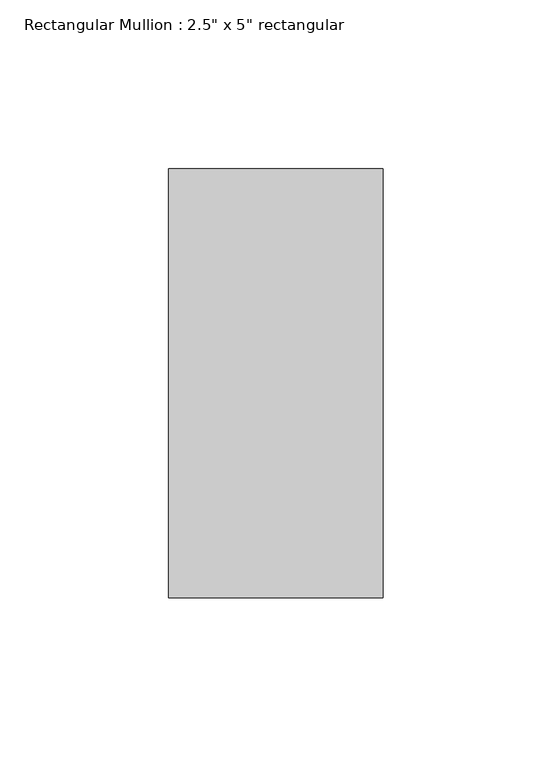
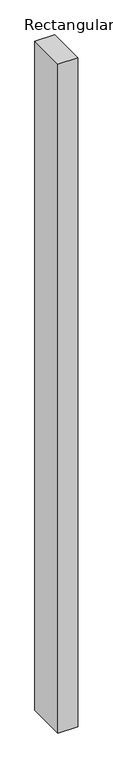
"""IFC4 building model written with IfcOpenShell, lengths in millimetres: member geometry."""

from ifc_helpers import new_model, si_unit, frame, origin, place, context, project, spatial, polyline, outline, extrude, source, transform, mapped, element, save


def member_d9e57c59(model_context):
    return source(origin(), model_context, "Body", "SweptSolid", [
        extrude(outline(polyline([(0.0, 63.5), (0.0, -63.5), (-63.5, -63.5), (-63.5, 63.5), (0.0, 63.5)])), frame((0.0, 0.0, -2256.3666667), z_axis=(0.0, 0.0, 1.0), x_axis=(1.0, 0.0, 0.0)), (0.0, 0.0, 1.0), 2256.3666667),
    ])


if __name__ == "__main__":
    model = new_model("IFC4")
    model_context = context("Model", 3, world=origin())
    ifc_project = project(units=[si_unit("LENGTHUNIT", "METRE", prefix="MILLI")], contexts=[model_context])
    site = spatial("IfcSite", under=ifc_project)
    building = spatial("IfcBuilding", under=site)
    placement = place(None, origin())
    member_shape = member_d9e57c59(model_context)
    element("IfcMember", 1, ObjectType="Rectangular Mullion : 2.5\" x 5\" rectangular", at=placement, inside=building, context=model_context, shape_type="MappedRepresentation", body=[
        mapped(member_shape, transform((0.0, 0.0, 0.0), x_axis=(1.0, 0.0, 0.0), y_axis=(0.0, 1.0, 0.0), z_axis=(0.0, 0.0, 1.0))),
    ])
    save(model, "model.ifc")

# Revit data of these elements
# Type "Rectangular Mullion : 2.5\" x 5\" rectangular"
#   built-in parameter 1007304 = 0.416667 (stored number, unit not read)
#   built-in parameter 1007301 = 0.104167 (stored number, unit not read)
#   built-in parameter 1007300 = 0.104167 (stored number, unit not read)
# Element 1 (IfcMember, "Rectangular Mullion : 2.5\" x 5\" rectangular")
#   Materials on its faces: "Aluminum"
# Materials
#   "Aluminum": class "Metal", colour RGB 247 247 247, transparency 0, Description = "Aluminum 6061", Cost = 0
